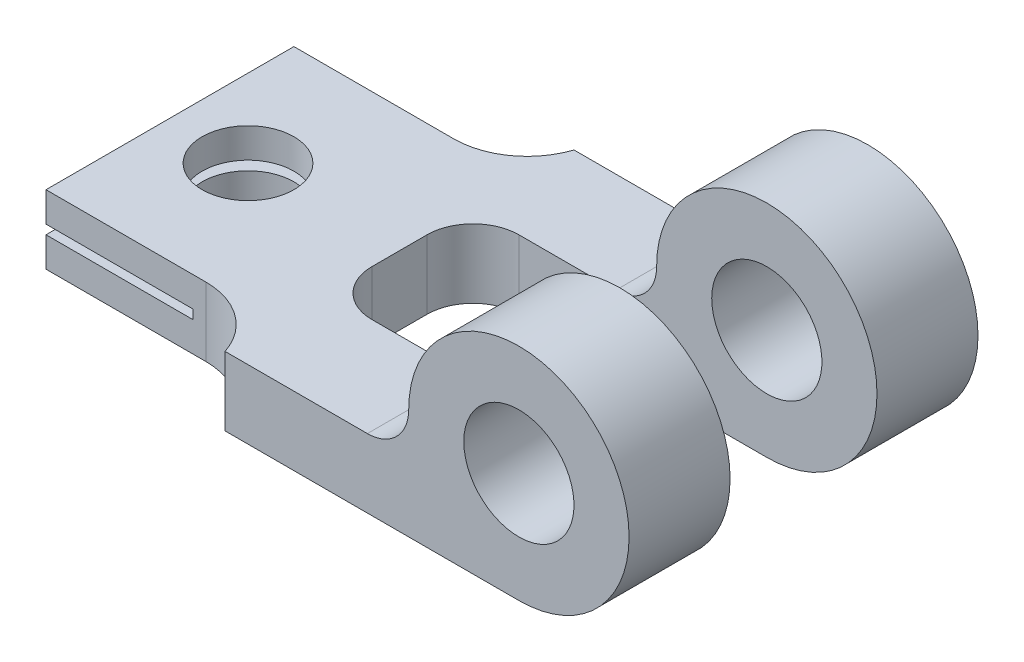
ISO-10303-21;
HEADER;
FILE_DESCRIPTION(('STEP AP214'),'2;1');
FILE_NAME('part.step','',(''),(''),'','','');
FILE_SCHEMA(('AUTOMOTIVE_DESIGN { 1 0 10303 214 1 1 1 1 }'));
ENDSEC;
DATA;
#1=APPLICATION_CONTEXT('core data for automotive mechanical design processes');
#2=APPLICATION_PROTOCOL_DEFINITION('international standard','automotive_design',2000,#1);
#3=PRODUCT_CONTEXT('',#1,'mechanical');
#4=PRODUCT('Part','Part','',(#3));
#5=PRODUCT_RELATED_PRODUCT_CATEGORY('part','',(#4));
#6=PRODUCT_DEFINITION_FORMATION('','',#4);
#7=PRODUCT_DEFINITION_CONTEXT('part definition',#1,'design');
#8=PRODUCT_DEFINITION('design','',#6,#7);
#9=PRODUCT_DEFINITION_SHAPE('','',#8);
#10=(LENGTH_UNIT() NAMED_UNIT(*) SI_UNIT(.MILLI.,.METRE.));
#11=(NAMED_UNIT(*) PLANE_ANGLE_UNIT() SI_UNIT($,.RADIAN.));
#12=(NAMED_UNIT(*) SI_UNIT($,.STERADIAN.) SOLID_ANGLE_UNIT());
#13=UNCERTAINTY_MEASURE_WITH_UNIT(LENGTH_MEASURE(1.E-05),#10,'distance_accuracy_value','');
#14=(GEOMETRIC_REPRESENTATION_CONTEXT(3) GLOBAL_UNCERTAINTY_ASSIGNED_CONTEXT((#13)) GLOBAL_UNIT_ASSIGNED_CONTEXT((#10,
#11,#12)) REPRESENTATION_CONTEXT('',''));
#15=CARTESIAN_POINT('',(0.,0.,0.));
#16=DIRECTION('',(0.,0.,1.));
#17=DIRECTION('',(1.,0.,0.));
#18=AXIS2_PLACEMENT_3D('',#15,#16,#17);
#19=CARTESIAN_POINT('',(0.,0.,27.));
#20=DIRECTION('',(-1.,0.,0.));
#21=DIRECTION('',(0.,-1.,0.));
#22=AXIS2_PLACEMENT_3D('',#19,#20,#21);
#23=PLANE('',#22);
#24=DIRECTION('',(0.,0.,-1.));
#25=VECTOR('',#24,1.);
#26=CARTESIAN_POINT('',(0.,0.,27.));
#27=LINE('',#26,#25);
#28=CARTESIAN_POINT('',(0.,0.,6.));
#29=VERTEX_POINT('',#28);
#30=CARTESIAN_POINT('',(0.,0.,-6.));
#31=VERTEX_POINT('',#30);
#32=EDGE_CURVE('E240',#29,#31,#27,.T.);
#33=ORIENTED_EDGE('',*,*,#32,.T.);
#34=DIRECTION('',(0.,1.,0.));
#35=VECTOR('',#34,1.);
#36=CARTESIAN_POINT('',(0.,15.,-6.));
#37=LINE('',#36,#35);
#38=CARTESIAN_POINT('',(0.,15.,-6.));
#39=VERTEX_POINT('',#38);
#40=EDGE_CURVE('E219',#31,#39,#37,.T.);
#41=ORIENTED_EDGE('',*,*,#40,.T.);
#42=DIRECTION('',(0.,0.,-1.));
#43=VECTOR('',#42,1.);
#44=CARTESIAN_POINT('',(0.,15.,27.));
#45=LINE('',#44,#43);
#46=CARTESIAN_POINT('',(0.,15.,6.));
#47=VERTEX_POINT('',#46);
#48=EDGE_CURVE('E235',#47,#39,#45,.T.);
#49=ORIENTED_EDGE('',*,*,#48,.F.);
#50=DIRECTION('',(0.,1.,0.));
#51=VECTOR('',#50,1.);
#52=CARTESIAN_POINT('',(0.,0.,6.));
#53=LINE('',#52,#51);
#54=EDGE_CURVE('E211',#47,#29,#53,.F.);
#55=ORIENTED_EDGE('',*,*,#54,.T.);
#56=EDGE_LOOP('',(#33,#41,#49,#55));
#57=FACE_BOUND('',#56,.T.);
#58=ADVANCED_FACE('F41',(#57),#23,.F.);
#59=CARTESIAN_POINT('',(0.,6.49999999999999,27.));
#60=DIRECTION('',(0.,1.,0.));
#61=DIRECTION('',(-1.,0.,0.));
#62=AXIS2_PLACEMENT_3D('',#59,#60,#61);
#63=PLANE('',#62);
#64=CARTESIAN_POINT('',(-33.,6.5,0.));
#65=DIRECTION('',(0.,1.,0.));
#66=DIRECTION('',(-1.,0.,0.));
#67=AXIS2_PLACEMENT_3D('',#64,#65,#66);
#68=CIRCLE('',#67,10.);
#69=CARTESIAN_POINT('',(-43.,6.5,0.));
#70=VERTEX_POINT('',#69);
#71=EDGE_CURVE('E310',#70,#70,#68,.T.);
#72=ORIENTED_EDGE('',*,*,#71,.F.);
#73=EDGE_LOOP('',(#72));
#74=FACE_BOUND('',#73,.T.);
#75=DIRECTION('',(1.,0.,0.));
#76=VECTOR('',#75,1.);
#77=CARTESIAN_POINT('',(0.,6.49999999999999,-27.));
#78=LINE('',#77,#76);
#79=CARTESIAN_POINT('',(-50.,6.5,-27.));
#80=VERTEX_POINT('',#79);
#81=CARTESIAN_POINT('',(-18.,6.49999999999999,-27.));
#82=VERTEX_POINT('',#81);
#83=EDGE_CURVE('E309',#80,#82,#78,.T.);
#84=ORIENTED_EDGE('',*,*,#83,.F.);
#85=DIRECTION('',(0.,0.,-1.));
#86=VECTOR('',#85,1.);
#87=CARTESIAN_POINT('',(-50.,6.5,27.));
#88=LINE('',#87,#86);
#89=CARTESIAN_POINT('',(-50.,6.5,27.));
#90=VERTEX_POINT('',#89);
#91=EDGE_CURVE('E356',#90,#80,#88,.T.);
#92=ORIENTED_EDGE('',*,*,#91,.F.);
#93=DIRECTION('',(1.,0.,0.));
#94=VECTOR('',#93,1.);
#95=CARTESIAN_POINT('',(0.,6.49999999999999,27.));
#96=LINE('',#95,#94);
#97=CARTESIAN_POINT('',(-18.,6.49999999999999,27.));
#98=VERTEX_POINT('',#97);
#99=EDGE_CURVE('E311',#90,#98,#96,.T.);
#100=ORIENTED_EDGE('',*,*,#99,.T.);
#101=DIRECTION('',(0.,0.,-1.));
#102=VECTOR('',#101,1.);
#103=CARTESIAN_POINT('',(-18.,6.49999999999999,27.));
#104=LINE('',#103,#102);
#105=EDGE_CURVE('E327',#98,#82,#104,.T.);
#106=ORIENTED_EDGE('',*,*,#105,.T.);
#107=EDGE_LOOP('',(#84,#92,#100,#106));
#108=FACE_BOUND('',#107,.T.);
#109=ADVANCED_FACE('F408',(#74,#108),#63,.T.);
#110=CARTESIAN_POINT('',(-50.,0.,27.));
#111=DIRECTION('',(1.,0.,0.));
#112=DIRECTION('',(0.,0.,-1.));
#113=AXIS2_PLACEMENT_3D('',#110,#111,#112);
#114=PLANE('',#113);
#115=DIRECTION('',(0.,-1.,0.));
#116=VECTOR('',#115,1.);
#117=CARTESIAN_POINT('',(-50.,0.,-27.));
#118=LINE('',#117,#116);
#119=CARTESIAN_POINT('',(-50.,0.,-27.));
#120=VERTEX_POINT('',#119);
#121=EDGE_CURVE('E332',#80,#120,#118,.T.);
#122=ORIENTED_EDGE('',*,*,#121,.T.);
#123=DIRECTION('',(0.,0.,-1.));
#124=VECTOR('',#123,1.);
#125=CARTESIAN_POINT('',(-50.,0.,27.));
#126=LINE('',#125,#124);
#127=CARTESIAN_POINT('',(-50.,0.,27.));
#128=VERTEX_POINT('',#127);
#129=EDGE_CURVE('E354',#128,#120,#126,.T.);
#130=ORIENTED_EDGE('',*,*,#129,.F.);
#131=DIRECTION('',(0.,-1.,0.));
#132=VECTOR('',#131,1.);
#133=CARTESIAN_POINT('',(-50.,0.,27.));
#134=LINE('',#133,#132);
#135=EDGE_CURVE('E313',#90,#128,#134,.T.);
#136=ORIENTED_EDGE('',*,*,#135,.F.);
#137=ORIENTED_EDGE('',*,*,#91,.T.);
#138=EDGE_LOOP('',(#122,#130,#136,#137));
#139=FACE_BOUND('',#138,.T.);
#140=ADVANCED_FACE('F420',(#139),#114,.F.);
#141=CARTESIAN_POINT('',(0.,0.,27.));
#142=DIRECTION('',(0.,1.,0.));
#143=DIRECTION('',(0.,0.,1.));
#144=AXIS2_PLACEMENT_3D('',#141,#142,#143);
#145=PLANE('',#144);
#146=CARTESIAN_POINT('',(-33.,0.,0.));
#147=DIRECTION('',(0.,1.,0.));
#148=DIRECTION('',(-1.,0.,0.));
#149=AXIS2_PLACEMENT_3D('',#146,#147,#148);
#150=CIRCLE('',#149,10.);
#151=CARTESIAN_POINT('',(-43.,0.,0.));
#152=VERTEX_POINT('',#151);
#153=EDGE_CURVE('E301',#152,#152,#150,.T.);
#154=ORIENTED_EDGE('',*,*,#153,.T.);
#155=EDGE_LOOP('',(#154));
#156=FACE_BOUND('',#155,.T.);
#157=DIRECTION('',(1.,0.,0.));
#158=VECTOR('',#157,1.);
#159=CARTESIAN_POINT('',(0.,0.,-27.));
#160=LINE('',#159,#158);
#161=CARTESIAN_POINT('',(-15.1986841535707,0.,-27.));
#162=VERTEX_POINT('',#161);
#163=EDGE_CURVE('E334',#120,#162,#160,.T.);
#164=ORIENTED_EDGE('',*,*,#163,.T.);
#165=CARTESIAN_POINT('',(-15.1986841535707,0.,-43.));
#166=DIRECTION('',(0.,1.,0.));
#167=DIRECTION('',(0.,0.,1.));
#168=AXIS2_PLACEMENT_3D('',#165,#166,#167);
#169=CIRCLE('',#168,16.);
#170=CARTESIAN_POINT('',(0.,0.,-38.));
#171=VERTEX_POINT('',#170);
#172=EDGE_CURVE('E210',#162,#171,#169,.T.);
#173=ORIENTED_EDGE('',*,*,#172,.T.);
#174=DIRECTION('',(-1.,0.,0.));
#175=VECTOR('',#174,1.);
#176=CARTESIAN_POINT('',(0.,0.,-38.));
#177=LINE('',#176,#175);
#178=CARTESIAN_POINT('',(64.,0.,-38.));
#179=VERTEX_POINT('',#178);
#180=EDGE_CURVE('E284',#179,#171,#177,.T.);
#181=ORIENTED_EDGE('',*,*,#180,.F.);
#182=DIRECTION('',(0.,0.,1.));
#183=VECTOR('',#182,1.);
#184=CARTESIAN_POINT('',(64.,0.,-38.));
#185=LINE('',#184,#183);
#186=CARTESIAN_POINT('',(64.,0.,-16.));
#187=VERTEX_POINT('',#186);
#188=EDGE_CURVE('E283',#179,#187,#185,.T.);
#189=ORIENTED_EDGE('',*,*,#188,.T.);
#190=DIRECTION('',(-1.,0.,0.));
#191=VECTOR('',#190,1.);
#192=CARTESIAN_POINT('',(0.,0.,-16.));
#193=LINE('',#192,#191);
#194=CARTESIAN_POINT('',(10.,0.,-16.));
#195=VERTEX_POINT('',#194);
#196=EDGE_CURVE('E273',#187,#195,#193,.T.);
#197=ORIENTED_EDGE('',*,*,#196,.T.);
#198=CARTESIAN_POINT('',(10.,0.,-6.));
#199=DIRECTION('',(0.,1.,0.));
#200=DIRECTION('',(0.,0.,1.));
#201=AXIS2_PLACEMENT_3D('',#198,#199,#200);
#202=CIRCLE('',#201,10.);
#203=EDGE_CURVE('E224',#195,#31,#202,.T.);
#204=ORIENTED_EDGE('',*,*,#203,.T.);
#205=ORIENTED_EDGE('',*,*,#32,.F.);
#206=CARTESIAN_POINT('',(10.,0.,6.));
#207=DIRECTION('',(0.,1.,0.));
#208=DIRECTION('',(0.,0.,1.));
#209=AXIS2_PLACEMENT_3D('',#206,#207,#208);
#210=CIRCLE('',#209,10.);
#211=CARTESIAN_POINT('',(10.,0.,16.));
#212=VERTEX_POINT('',#211);
#213=EDGE_CURVE('E11',#29,#212,#210,.T.);
#214=ORIENTED_EDGE('',*,*,#213,.T.);
#215=DIRECTION('',(-1.,0.,0.));
#216=VECTOR('',#215,1.);
#217=CARTESIAN_POINT('',(0.,0.,16.));
#218=LINE('',#217,#216);
#219=CARTESIAN_POINT('',(64.,0.,16.));
#220=VERTEX_POINT('',#219);
#221=EDGE_CURVE('E242',#220,#212,#218,.T.);
#222=ORIENTED_EDGE('',*,*,#221,.F.);
#223=DIRECTION('',(0.,0.,-1.));
#224=VECTOR('',#223,1.);
#225=CARTESIAN_POINT('',(64.,0.,38.));
#226=LINE('',#225,#224);
#227=CARTESIAN_POINT('',(64.,0.,38.));
#228=VERTEX_POINT('',#227);
#229=EDGE_CURVE('E196',#228,#220,#226,.T.);
#230=ORIENTED_EDGE('',*,*,#229,.F.);
#231=DIRECTION('',(-1.,0.,0.));
#232=VECTOR('',#231,1.);
#233=CARTESIAN_POINT('',(0.,0.,38.));
#234=LINE('',#233,#232);
#235=CARTESIAN_POINT('',(0.,0.,38.));
#236=VERTEX_POINT('',#235);
#237=EDGE_CURVE('E182',#228,#236,#234,.T.);
#238=ORIENTED_EDGE('',*,*,#237,.T.);
#239=CARTESIAN_POINT('',(-15.1986841535707,0.,43.));
#240=DIRECTION('',(0.,1.,0.));
#241=DIRECTION('',(0.,0.,1.));
#242=AXIS2_PLACEMENT_3D('',#239,#240,#241);
#243=CIRCLE('',#242,16.);
#244=CARTESIAN_POINT('',(-15.1986841535707,0.,27.));
#245=VERTEX_POINT('',#244);
#246=EDGE_CURVE('E193',#236,#245,#243,.T.);
#247=ORIENTED_EDGE('',*,*,#246,.T.);
#248=DIRECTION('',(1.,0.,0.));
#249=VECTOR('',#248,1.);
#250=CARTESIAN_POINT('',(0.,0.,27.));
#251=LINE('',#250,#249);
#252=EDGE_CURVE('E320',#128,#245,#251,.T.);
#253=ORIENTED_EDGE('',*,*,#252,.F.);
#254=ORIENTED_EDGE('',*,*,#129,.T.);
#255=EDGE_LOOP('',(#164,#173,#181,#189,#197,#204,#205,#214,#222,#230,#238,#247,#253,#254));
#256=FACE_BOUND('',#255,.T.);
#257=ADVANCED_FACE('F194',(#156,#256),#145,.F.);
#258=CARTESIAN_POINT('',(0.,15.,27.));
#259=DIRECTION('',(0.,-1.,0.));
#260=DIRECTION('',(1.,0.,0.));
#261=AXIS2_PLACEMENT_3D('',#258,#259,#260);
#262=PLANE('',#261);
#263=CARTESIAN_POINT('',(-33.,15.,0.));
#264=DIRECTION('',(0.,1.,0.));
#265=DIRECTION('',(-1.,0.,0.));
#266=AXIS2_PLACEMENT_3D('',#263,#264,#265);
#267=CIRCLE('',#266,10.);
#268=CARTESIAN_POINT('',(-43.,15.,0.));
#269=VERTEX_POINT('',#268);
#270=EDGE_CURVE('E297',#269,#269,#267,.T.);
#271=ORIENTED_EDGE('',*,*,#270,.F.);
#272=EDGE_LOOP('',(#271));
#273=FACE_BOUND('',#272,.T.);
#274=DIRECTION('',(1.,0.,0.));
#275=VECTOR('',#274,1.);
#276=CARTESIAN_POINT('',(0.,15.,-38.));
#277=LINE('',#276,#275);
#278=CARTESIAN_POINT('',(0.,15.,-38.));
#279=VERTEX_POINT('',#278);
#280=CARTESIAN_POINT('',(31.,15.,-38.));
#281=VERTEX_POINT('',#280);
#282=EDGE_CURVE('E274',#279,#281,#277,.T.);
#283=ORIENTED_EDGE('',*,*,#282,.F.);
#284=CARTESIAN_POINT('',(-15.1986841535707,15.,-43.));
#285=DIRECTION('',(0.,-1.,0.));
#286=DIRECTION('',(1.,0.,0.));
#287=AXIS2_PLACEMENT_3D('',#284,#285,#286);
#288=CIRCLE('',#287,16.);
#289=CARTESIAN_POINT('',(-15.1986841535707,15.,-27.));
#290=VERTEX_POINT('',#289);
#291=EDGE_CURVE('E203',#279,#290,#288,.T.);
#292=ORIENTED_EDGE('',*,*,#291,.T.);
#293=DIRECTION('',(-1.,0.,0.));
#294=VECTOR('',#293,1.);
#295=CARTESIAN_POINT('',(0.,15.,-27.));
#296=LINE('',#295,#294);
#297=CARTESIAN_POINT('',(-50.,15.,-27.));
#298=VERTEX_POINT('',#297);
#299=EDGE_CURVE('E340',#290,#298,#296,.T.);
#300=ORIENTED_EDGE('',*,*,#299,.T.);
#301=DIRECTION('',(0.,0.,-1.));
#302=VECTOR('',#301,1.);
#303=CARTESIAN_POINT('',(-50.,15.,27.));
#304=LINE('',#303,#302);
#305=CARTESIAN_POINT('',(-50.,15.,27.));
#306=VERTEX_POINT('',#305);
#307=EDGE_CURVE('E238',#306,#298,#304,.T.);
#308=ORIENTED_EDGE('',*,*,#307,.F.);
#309=DIRECTION('',(-1.,0.,0.));
#310=VECTOR('',#309,1.);
#311=CARTESIAN_POINT('',(0.,15.,27.));
#312=LINE('',#311,#310);
#313=CARTESIAN_POINT('',(-15.1986841535707,15.,27.));
#314=VERTEX_POINT('',#313);
#315=EDGE_CURVE('E316',#314,#306,#312,.T.);
#316=ORIENTED_EDGE('',*,*,#315,.F.);
#317=CARTESIAN_POINT('',(-15.1986841535707,15.,43.));
#318=DIRECTION('',(0.,-1.,0.));
#319=DIRECTION('',(1.,0.,0.));
#320=AXIS2_PLACEMENT_3D('',#317,#318,#319);
#321=CIRCLE('',#320,16.);
#322=CARTESIAN_POINT('',(0.,15.,38.));
#323=VERTEX_POINT('',#322);
#324=EDGE_CURVE('E204',#314,#323,#321,.T.);
#325=ORIENTED_EDGE('',*,*,#324,.T.);
#326=DIRECTION('',(1.,0.,0.));
#327=VECTOR('',#326,1.);
#328=CARTESIAN_POINT('',(0.,15.,38.));
#329=LINE('',#328,#327);
#330=CARTESIAN_POINT('',(31.,15.,38.));
#331=VERTEX_POINT('',#330);
#332=EDGE_CURVE('E190',#323,#331,#329,.T.);
#333=ORIENTED_EDGE('',*,*,#332,.T.);
#334=DIRECTION('',(0.,0.,-1.));
#335=VECTOR('',#334,1.);
#336=CARTESIAN_POINT('',(31.,15.,38.));
#337=LINE('',#336,#335);
#338=CARTESIAN_POINT('',(31.,15.,16.));
#339=VERTEX_POINT('',#338);
#340=EDGE_CURVE('E256',#331,#339,#337,.T.);
#341=ORIENTED_EDGE('',*,*,#340,.T.);
#342=DIRECTION('',(1.,0.,0.));
#343=VECTOR('',#342,1.);
#344=CARTESIAN_POINT('',(0.,15.,16.));
#345=LINE('',#344,#343);
#346=CARTESIAN_POINT('',(10.,15.,16.));
#347=VERTEX_POINT('',#346);
#348=EDGE_CURVE('E188',#347,#339,#345,.T.);
#349=ORIENTED_EDGE('',*,*,#348,.F.);
#350=CARTESIAN_POINT('',(10.,15.,6.));
#351=DIRECTION('',(0.,-1.,0.));
#352=DIRECTION('',(1.,0.,0.));
#353=AXIS2_PLACEMENT_3D('',#350,#351,#352);
#354=CIRCLE('',#353,10.);
#355=EDGE_CURVE('E47',#347,#47,#354,.T.);
#356=ORIENTED_EDGE('',*,*,#355,.T.);
#357=ORIENTED_EDGE('',*,*,#48,.T.);
#358=CARTESIAN_POINT('',(10.,15.,-6.));
#359=DIRECTION('',(0.,-1.,0.));
#360=DIRECTION('',(1.,0.,0.));
#361=AXIS2_PLACEMENT_3D('',#358,#359,#360);
#362=CIRCLE('',#361,10.);
#363=CARTESIAN_POINT('',(10.,15.,-16.));
#364=VERTEX_POINT('',#363);
#365=EDGE_CURVE('E222',#39,#364,#362,.T.);
#366=ORIENTED_EDGE('',*,*,#365,.T.);
#367=DIRECTION('',(1.,0.,0.));
#368=VECTOR('',#367,1.);
#369=CARTESIAN_POINT('',(0.,15.,-16.));
#370=LINE('',#369,#368);
#371=CARTESIAN_POINT('',(31.,15.,-16.));
#372=VERTEX_POINT('',#371);
#373=EDGE_CURVE('E267',#364,#372,#370,.T.);
#374=ORIENTED_EDGE('',*,*,#373,.T.);
#375=DIRECTION('',(0.,0.,1.));
#376=VECTOR('',#375,1.);
#377=CARTESIAN_POINT('',(31.,15.,-38.));
#378=LINE('',#377,#376);
#379=EDGE_CURVE('E300',#281,#372,#378,.T.);
#380=ORIENTED_EDGE('',*,*,#379,.F.);
#381=EDGE_LOOP('',(#283,#292,#300,#308,#316,#325,#333,#341,#349,#356,#357,#366,#374,#380));
#382=FACE_BOUND('',#381,.T.);
#383=ADVANCED_FACE('F233',(#273,#382),#262,.F.);
#384=CARTESIAN_POINT('',(-50.,0.,27.));
#385=DIRECTION('',(-1.,0.,0.));
#386=DIRECTION('',(0.,0.,1.));
#387=AXIS2_PLACEMENT_3D('',#384,#385,#386);
#388=PLANE('',#387);
#389=DIRECTION('',(0.,1.,0.));
#390=VECTOR('',#389,1.);
#391=CARTESIAN_POINT('',(-50.,0.,-27.));
#392=LINE('',#391,#390);
#393=CARTESIAN_POINT('',(-50.,8.49999999999999,-27.));
#394=VERTEX_POINT('',#393);
#395=EDGE_CURVE('E339',#394,#298,#392,.T.);
#396=ORIENTED_EDGE('',*,*,#395,.F.);
#397=DIRECTION('',(0.,0.,-1.));
#398=VECTOR('',#397,1.);
#399=CARTESIAN_POINT('',(-50.,8.49999999999999,27.));
#400=LINE('',#399,#398);
#401=CARTESIAN_POINT('',(-50.,8.49999999999999,27.));
#402=VERTEX_POINT('',#401);
#403=EDGE_CURVE('E347',#402,#394,#400,.T.);
#404=ORIENTED_EDGE('',*,*,#403,.F.);
#405=DIRECTION('',(0.,1.,0.));
#406=VECTOR('',#405,1.);
#407=CARTESIAN_POINT('',(-50.,0.,27.));
#408=LINE('',#407,#406);
#409=EDGE_CURVE('E322',#402,#306,#408,.T.);
#410=ORIENTED_EDGE('',*,*,#409,.T.);
#411=ORIENTED_EDGE('',*,*,#307,.T.);
#412=EDGE_LOOP('',(#396,#404,#410,#411));
#413=FACE_BOUND('',#412,.T.);
#414=ADVANCED_FACE('F515',(#413),#388,.T.);
#415=CARTESIAN_POINT('',(0.,8.5,27.));
#416=DIRECTION('',(0.,-1.,0.));
#417=DIRECTION('',(1.,0.,0.));
#418=AXIS2_PLACEMENT_3D('',#415,#416,#417);
#419=PLANE('',#418);
#420=CARTESIAN_POINT('',(-33.,8.5,0.));
#421=DIRECTION('',(0.,-1.,0.));
#422=DIRECTION('',(1.,0.,0.));
#423=AXIS2_PLACEMENT_3D('',#420,#421,#422);
#424=CIRCLE('',#423,10.);
#425=CARTESIAN_POINT('',(-23.,8.5,0.));
#426=VERTEX_POINT('',#425);
#427=EDGE_CURVE('E302',#426,#426,#424,.T.);
#428=ORIENTED_EDGE('',*,*,#427,.F.);
#429=EDGE_LOOP('',(#428));
#430=FACE_BOUND('',#429,.T.);
#431=DIRECTION('',(-1.,0.,0.));
#432=VECTOR('',#431,1.);
#433=CARTESIAN_POINT('',(0.,8.5,-27.));
#434=LINE('',#433,#432);
#435=CARTESIAN_POINT('',(-18.,8.5,-27.));
#436=VERTEX_POINT('',#435);
#437=EDGE_CURVE('E345',#436,#394,#434,.T.);
#438=ORIENTED_EDGE('',*,*,#437,.F.);
#439=DIRECTION('',(0.,0.,-1.));
#440=VECTOR('',#439,1.);
#441=CARTESIAN_POINT('',(-18.,8.5,27.));
#442=LINE('',#441,#440);
#443=CARTESIAN_POINT('',(-18.,8.5,27.));
#444=VERTEX_POINT('',#443);
#445=EDGE_CURVE('E350',#444,#436,#442,.T.);
#446=ORIENTED_EDGE('',*,*,#445,.F.);
#447=DIRECTION('',(-1.,0.,0.));
#448=VECTOR('',#447,1.);
#449=CARTESIAN_POINT('',(0.,8.5,27.));
#450=LINE('',#449,#448);
#451=EDGE_CURVE('E321',#444,#402,#450,.T.);
#452=ORIENTED_EDGE('',*,*,#451,.T.);
#453=ORIENTED_EDGE('',*,*,#403,.T.);
#454=EDGE_LOOP('',(#438,#446,#452,#453));
#455=FACE_BOUND('',#454,.T.);
#456=ADVANCED_FACE('F586',(#430,#455),#419,.T.);
#457=CARTESIAN_POINT('',(-18.,0.,27.));
#458=DIRECTION('',(-1.,0.,0.));
#459=DIRECTION('',(0.,0.,1.));
#460=AXIS2_PLACEMENT_3D('',#457,#458,#459);
#461=PLANE('',#460);
#462=DIRECTION('',(0.,1.,0.));
#463=VECTOR('',#462,1.);
#464=CARTESIAN_POINT('',(-18.,0.,-27.));
#465=LINE('',#464,#463);
#466=EDGE_CURVE('E314',#82,#436,#465,.T.);
#467=ORIENTED_EDGE('',*,*,#466,.F.);
#468=ORIENTED_EDGE('',*,*,#105,.F.);
#469=DIRECTION('',(0.,1.,0.));
#470=VECTOR('',#469,1.);
#471=CARTESIAN_POINT('',(-18.,0.,27.));
#472=LINE('',#471,#470);
#473=EDGE_CURVE('E326',#98,#444,#472,.T.);
#474=ORIENTED_EDGE('',*,*,#473,.T.);
#475=ORIENTED_EDGE('',*,*,#445,.T.);
#476=EDGE_LOOP('',(#467,#468,#474,#475));
#477=FACE_BOUND('',#476,.T.);
#478=ADVANCED_FACE('F573',(#477),#461,.T.);
#479=CARTESIAN_POINT('',(0.,0.,27.));
#480=DIRECTION('',(0.,0.,1.));
#481=DIRECTION('',(1.,0.,0.));
#482=AXIS2_PLACEMENT_3D('',#479,#480,#481);
#483=PLANE('',#482);
#484=ORIENTED_EDGE('',*,*,#252,.T.);
#485=DIRECTION('',(0.,-1.,0.));
#486=VECTOR('',#485,1.);
#487=CARTESIAN_POINT('',(-15.1986841535707,15.,27.));
#488=LINE('',#487,#486);
#489=EDGE_CURVE('E202',#245,#314,#488,.F.);
#490=ORIENTED_EDGE('',*,*,#489,.T.);
#491=ORIENTED_EDGE('',*,*,#315,.T.);
#492=ORIENTED_EDGE('',*,*,#409,.F.);
#493=ORIENTED_EDGE('',*,*,#451,.F.);
#494=ORIENTED_EDGE('',*,*,#473,.F.);
#495=ORIENTED_EDGE('',*,*,#99,.F.);
#496=ORIENTED_EDGE('',*,*,#135,.T.);
#497=EDGE_LOOP('',(#484,#490,#491,#492,#493,#494,#495,#496));
#498=FACE_BOUND('',#497,.T.);
#499=ADVANCED_FACE('F566',(#498),#483,.T.);
#500=CARTESIAN_POINT('',(0.,0.,-27.));
#501=DIRECTION('',(0.,0.,1.));
#502=DIRECTION('',(1.,0.,0.));
#503=AXIS2_PLACEMENT_3D('',#500,#501,#502);
#504=PLANE('',#503);
#505=ORIENTED_EDGE('',*,*,#299,.F.);
#506=DIRECTION('',(0.,1.,0.));
#507=VECTOR('',#506,1.);
#508=CARTESIAN_POINT('',(-15.1986841535707,0.,-27.));
#509=LINE('',#508,#507);
#510=EDGE_CURVE('E209',#290,#162,#509,.F.);
#511=ORIENTED_EDGE('',*,*,#510,.T.);
#512=ORIENTED_EDGE('',*,*,#163,.F.);
#513=ORIENTED_EDGE('',*,*,#121,.F.);
#514=ORIENTED_EDGE('',*,*,#83,.T.);
#515=ORIENTED_EDGE('',*,*,#466,.T.);
#516=ORIENTED_EDGE('',*,*,#437,.T.);
#517=ORIENTED_EDGE('',*,*,#395,.T.);
#518=EDGE_LOOP('',(#505,#511,#512,#513,#514,#515,#516,#517));
#519=FACE_BOUND('',#518,.T.);
#520=ADVANCED_FACE('F366',(#519),#504,.F.);
#521=CARTESIAN_POINT('',(-33.,0.,0.));
#522=DIRECTION('',(0.,1.,0.));
#523=DIRECTION('',(-1.,0.,0.));
#524=AXIS2_PLACEMENT_3D('',#521,#522,#523);
#525=CYLINDRICAL_SURFACE('',#524,10.);
#526=ORIENTED_EDGE('',*,*,#427,.T.);
#527=EDGE_LOOP('',(#526));
#528=FACE_BOUND('',#527,.T.);
#529=ORIENTED_EDGE('',*,*,#270,.T.);
#530=EDGE_LOOP('',(#529));
#531=FACE_BOUND('',#530,.T.);
#532=ADVANCED_FACE('F564',(#528,#531),#525,.F.);
#533=ORIENTED_EDGE('',*,*,#71,.T.);
#534=EDGE_LOOP('',(#533));
#535=FACE_BOUND('',#534,.T.);
#536=ORIENTED_EDGE('',*,*,#153,.F.);
#537=EDGE_LOOP('',(#536));
#538=FACE_BOUND('',#537,.T.);
#539=ADVANCED_FACE('F560',(#535,#538),#525,.F.);
#540=CARTESIAN_POINT('',(31.,24.,-38.));
#541=DIRECTION('',(0.,0.,-1.));
#542=DIRECTION('',(-1.,0.,0.));
#543=AXIS2_PLACEMENT_3D('',#540,#541,#542);
#544=PLANE('',#543);
#545=DIRECTION('',(0.,1.,0.));
#546=VECTOR('',#545,1.);
#547=CARTESIAN_POINT('',(0.,0.,-38.));
#548=LINE('',#547,#546);
#549=EDGE_CURVE('E272',#171,#279,#548,.T.);
#550=ORIENTED_EDGE('',*,*,#549,.T.);
#551=ORIENTED_EDGE('',*,*,#282,.T.);
#552=CARTESIAN_POINT('',(31.,24.,-38.));
#553=DIRECTION('',(0.,0.,1.));
#554=DIRECTION('',(-1.,0.,0.));
#555=AXIS2_PLACEMENT_3D('',#552,#553,#554);
#556=CIRCLE('',#555,9.00000000000001);
#557=CARTESIAN_POINT('',(40.,24.,-38.));
#558=VERTEX_POINT('',#557);
#559=EDGE_CURVE('E280',#281,#558,#556,.T.);
#560=ORIENTED_EDGE('',*,*,#559,.T.);
#561=CARTESIAN_POINT('',(64.,24.,-38.));
#562=DIRECTION('',(0.,0.,-1.));
#563=DIRECTION('',(-1.,0.,0.));
#564=AXIS2_PLACEMENT_3D('',#561,#562,#563);
#565=CIRCLE('',#564,24.);
#566=EDGE_CURVE('E276',#558,#179,#565,.T.);
#567=ORIENTED_EDGE('',*,*,#566,.T.);
#568=ORIENTED_EDGE('',*,*,#180,.T.);
#569=EDGE_LOOP('',(#550,#551,#560,#567,#568));
#570=FACE_BOUND('',#569,.T.);
#571=CARTESIAN_POINT('',(64.,24.,-38.));
#572=DIRECTION('',(0.,0.,-1.));
#573=DIRECTION('',(-1.,0.,0.));
#574=AXIS2_PLACEMENT_3D('',#571,#572,#573);
#575=CIRCLE('',#574,12.);
#576=CARTESIAN_POINT('',(52.,24.,-38.));
#577=VERTEX_POINT('',#576);
#578=EDGE_CURVE('E262',#577,#577,#575,.T.);
#579=ORIENTED_EDGE('',*,*,#578,.F.);
#580=EDGE_LOOP('',(#579));
#581=FACE_BOUND('',#580,.T.);
#582=ADVANCED_FACE('F374',(#570,#581),#544,.T.);
#583=CARTESIAN_POINT('',(31.,24.,-16.));
#584=DIRECTION('',(0.,0.,-1.));
#585=DIRECTION('',(-1.,0.,0.));
#586=AXIS2_PLACEMENT_3D('',#583,#584,#585);
#587=PLANE('',#586);
#588=ORIENTED_EDGE('',*,*,#373,.F.);
#589=DIRECTION('',(0.,1.,0.));
#590=VECTOR('',#589,1.);
#591=CARTESIAN_POINT('',(10.,0.,-16.));
#592=LINE('',#591,#590);
#593=EDGE_CURVE('E218',#364,#195,#592,.F.);
#594=ORIENTED_EDGE('',*,*,#593,.T.);
#595=ORIENTED_EDGE('',*,*,#196,.F.);
#596=CARTESIAN_POINT('',(64.,24.,-16.));
#597=DIRECTION('',(0.,0.,-1.));
#598=DIRECTION('',(-1.,0.,0.));
#599=AXIS2_PLACEMENT_3D('',#596,#597,#598);
#600=CIRCLE('',#599,24.);
#601=CARTESIAN_POINT('',(40.,24.,-16.));
#602=VERTEX_POINT('',#601);
#603=EDGE_CURVE('E287',#602,#187,#600,.T.);
#604=ORIENTED_EDGE('',*,*,#603,.F.);
#605=CARTESIAN_POINT('',(31.,24.,-16.));
#606=DIRECTION('',(0.,0.,1.));
#607=DIRECTION('',(-1.,0.,0.));
#608=AXIS2_PLACEMENT_3D('',#605,#606,#607);
#609=CIRCLE('',#608,9.00000000000001);
#610=EDGE_CURVE('E286',#372,#602,#609,.T.);
#611=ORIENTED_EDGE('',*,*,#610,.F.);
#612=EDGE_LOOP('',(#588,#594,#595,#604,#611));
#613=FACE_BOUND('',#612,.T.);
#614=CARTESIAN_POINT('',(64.,24.,-16.));
#615=DIRECTION('',(0.,0.,-1.));
#616=DIRECTION('',(-1.,0.,0.));
#617=AXIS2_PLACEMENT_3D('',#614,#615,#616);
#618=CIRCLE('',#617,12.);
#619=CARTESIAN_POINT('',(52.,24.,-16.));
#620=VERTEX_POINT('',#619);
#621=EDGE_CURVE('E263',#620,#620,#618,.T.);
#622=ORIENTED_EDGE('',*,*,#621,.T.);
#623=EDGE_LOOP('',(#622));
#624=FACE_BOUND('',#623,.T.);
#625=ADVANCED_FACE('F387',(#613,#624),#587,.F.);
#626=CARTESIAN_POINT('',(31.,24.,-38.));
#627=DIRECTION('',(0.,0.,1.));
#628=DIRECTION('',(1.,0.,0.));
#629=AXIS2_PLACEMENT_3D('',#626,#627,#628);
#630=CYLINDRICAL_SURFACE('',#629,9.00000000000001);
#631=ORIENTED_EDGE('',*,*,#610,.T.);
#632=DIRECTION('',(0.,0.,1.));
#633=VECTOR('',#632,1.);
#634=CARTESIAN_POINT('',(40.,24.,-38.));
#635=LINE('',#634,#633);
#636=EDGE_CURVE('E295',#558,#602,#635,.T.);
#637=ORIENTED_EDGE('',*,*,#636,.F.);
#638=ORIENTED_EDGE('',*,*,#559,.F.);
#639=ORIENTED_EDGE('',*,*,#379,.T.);
#640=EDGE_LOOP('',(#631,#637,#638,#639));
#641=FACE_BOUND('',#640,.T.);
#642=ADVANCED_FACE('F393',(#641),#630,.F.);
#643=CARTESIAN_POINT('',(64.,24.,-38.));
#644=DIRECTION('',(0.,0.,1.));
#645=DIRECTION('',(1.,0.,0.));
#646=AXIS2_PLACEMENT_3D('',#643,#644,#645);
#647=CYLINDRICAL_SURFACE('',#646,24.);
#648=ORIENTED_EDGE('',*,*,#603,.T.);
#649=ORIENTED_EDGE('',*,*,#188,.F.);
#650=ORIENTED_EDGE('',*,*,#566,.F.);
#651=ORIENTED_EDGE('',*,*,#636,.T.);
#652=EDGE_LOOP('',(#648,#649,#650,#651));
#653=FACE_BOUND('',#652,.T.);
#654=ADVANCED_FACE('F396',(#653),#647,.T.);
#655=CARTESIAN_POINT('',(64.,24.,-38.));
#656=DIRECTION('',(0.,0.,1.));
#657=DIRECTION('',(1.,0.,0.));
#658=AXIS2_PLACEMENT_3D('',#655,#656,#657);
#659=CYLINDRICAL_SURFACE('',#658,12.);
#660=ORIENTED_EDGE('',*,*,#578,.T.);
#661=EDGE_LOOP('',(#660));
#662=FACE_BOUND('',#661,.T.);
#663=ORIENTED_EDGE('',*,*,#621,.F.);
#664=EDGE_LOOP('',(#663));
#665=FACE_BOUND('',#664,.T.);
#666=ADVANCED_FACE('F397',(#662,#665),#659,.F.);
#667=CARTESIAN_POINT('',(64.,24.,38.));
#668=DIRECTION('',(0.,0.,-1.));
#669=DIRECTION('',(-1.,0.,0.));
#670=AXIS2_PLACEMENT_3D('',#667,#668,#669);
#671=CYLINDRICAL_SURFACE('',#670,24.);
#672=CARTESIAN_POINT('',(64.,24.,16.));
#673=DIRECTION('',(0.,0.,-1.));
#674=DIRECTION('',(-1.,0.,0.));
#675=AXIS2_PLACEMENT_3D('',#672,#673,#674);
#676=CIRCLE('',#675,24.);
#677=CARTESIAN_POINT('',(40.,24.,16.));
#678=VERTEX_POINT('',#677);
#679=EDGE_CURVE('E246',#678,#220,#676,.T.);
#680=ORIENTED_EDGE('',*,*,#679,.F.);
#681=DIRECTION('',(0.,0.,-1.));
#682=VECTOR('',#681,1.);
#683=CARTESIAN_POINT('',(40.,24.,38.));
#684=LINE('',#683,#682);
#685=CARTESIAN_POINT('',(40.,24.,38.));
#686=VERTEX_POINT('',#685);
#687=EDGE_CURVE('E264',#686,#678,#684,.T.);
#688=ORIENTED_EDGE('',*,*,#687,.F.);
#689=CARTESIAN_POINT('',(64.,24.,38.));
#690=DIRECTION('',(0.,0.,-1.));
#691=DIRECTION('',(-1.,0.,0.));
#692=AXIS2_PLACEMENT_3D('',#689,#690,#691);
#693=CIRCLE('',#692,24.);
#694=EDGE_CURVE('E200',#686,#228,#693,.T.);
#695=ORIENTED_EDGE('',*,*,#694,.T.);
#696=ORIENTED_EDGE('',*,*,#229,.T.);
#697=EDGE_LOOP('',(#680,#688,#695,#696));
#698=FACE_BOUND('',#697,.T.);
#699=ADVANCED_FACE('F404',(#698),#671,.T.);
#700=CARTESIAN_POINT('',(31.,24.,38.));
#701=DIRECTION('',(0.,0.,-1.));
#702=DIRECTION('',(-1.,0.,0.));
#703=AXIS2_PLACEMENT_3D('',#700,#701,#702);
#704=CYLINDRICAL_SURFACE('',#703,9.00000000000001);
#705=CARTESIAN_POINT('',(31.,24.,16.));
#706=DIRECTION('',(0.,0.,1.));
#707=DIRECTION('',(-1.,0.,0.));
#708=AXIS2_PLACEMENT_3D('',#705,#706,#707);
#709=CIRCLE('',#708,9.00000000000001);
#710=EDGE_CURVE('E248',#339,#678,#709,.T.);
#711=ORIENTED_EDGE('',*,*,#710,.F.);
#712=ORIENTED_EDGE('',*,*,#340,.F.);
#713=CARTESIAN_POINT('',(31.,24.,38.));
#714=DIRECTION('',(0.,0.,1.));
#715=DIRECTION('',(-1.,0.,0.));
#716=AXIS2_PLACEMENT_3D('',#713,#714,#715);
#717=CIRCLE('',#716,9.00000000000001);
#718=EDGE_CURVE('E648',#331,#686,#717,.T.);
#719=ORIENTED_EDGE('',*,*,#718,.T.);
#720=ORIENTED_EDGE('',*,*,#687,.T.);
#721=EDGE_LOOP('',(#711,#712,#719,#720));
#722=FACE_BOUND('',#721,.T.);
#723=ADVANCED_FACE('F483',(#722),#704,.F.);
#724=CARTESIAN_POINT('',(31.,24.,38.));
#725=DIRECTION('',(0.,0.,1.));
#726=DIRECTION('',(-1.,0.,0.));
#727=AXIS2_PLACEMENT_3D('',#724,#725,#726);
#728=PLANE('',#727);
#729=CARTESIAN_POINT('',(64.,24.,38.));
#730=DIRECTION('',(0.,0.,-1.));
#731=DIRECTION('',(-1.,0.,0.));
#732=AXIS2_PLACEMENT_3D('',#729,#730,#731);
#733=CIRCLE('',#732,12.);
#734=CARTESIAN_POINT('',(52.,24.,38.));
#735=VERTEX_POINT('',#734);
#736=EDGE_CURVE('E250',#735,#735,#733,.T.);
#737=ORIENTED_EDGE('',*,*,#736,.T.);
#738=EDGE_LOOP('',(#737));
#739=FACE_BOUND('',#738,.T.);
#740=DIRECTION('',(0.,1.,0.));
#741=VECTOR('',#740,1.);
#742=CARTESIAN_POINT('',(0.,0.,38.));
#743=LINE('',#742,#741);
#744=EDGE_CURVE('E177',#236,#323,#743,.T.);
#745=ORIENTED_EDGE('',*,*,#744,.F.);
#746=ORIENTED_EDGE('',*,*,#237,.F.);
#747=ORIENTED_EDGE('',*,*,#694,.F.);
#748=ORIENTED_EDGE('',*,*,#718,.F.);
#749=ORIENTED_EDGE('',*,*,#332,.F.);
#750=EDGE_LOOP('',(#745,#746,#747,#748,#749));
#751=FACE_BOUND('',#750,.T.);
#752=ADVANCED_FACE('F181',(#739,#751),#728,.T.);
#753=CARTESIAN_POINT('',(31.,24.,16.));
#754=DIRECTION('',(0.,0.,1.));
#755=DIRECTION('',(-1.,0.,0.));
#756=AXIS2_PLACEMENT_3D('',#753,#754,#755);
#757=PLANE('',#756);
#758=CARTESIAN_POINT('',(64.,24.,16.));
#759=DIRECTION('',(0.,0.,-1.));
#760=DIRECTION('',(-1.,0.,0.));
#761=AXIS2_PLACEMENT_3D('',#758,#759,#760);
#762=CIRCLE('',#761,12.);
#763=CARTESIAN_POINT('',(52.,24.,16.));
#764=VERTEX_POINT('',#763);
#765=EDGE_CURVE('E255',#764,#764,#762,.T.);
#766=ORIENTED_EDGE('',*,*,#765,.F.);
#767=EDGE_LOOP('',(#766));
#768=FACE_BOUND('',#767,.T.);
#769=ORIENTED_EDGE('',*,*,#221,.T.);
#770=DIRECTION('',(0.,1.,0.));
#771=VECTOR('',#770,1.);
#772=CARTESIAN_POINT('',(10.,15.,16.));
#773=LINE('',#772,#771);
#774=EDGE_CURVE('E221',#212,#347,#773,.T.);
#775=ORIENTED_EDGE('',*,*,#774,.T.);
#776=ORIENTED_EDGE('',*,*,#348,.T.);
#777=ORIENTED_EDGE('',*,*,#710,.T.);
#778=ORIENTED_EDGE('',*,*,#679,.T.);
#779=EDGE_LOOP('',(#769,#775,#776,#777,#778));
#780=FACE_BOUND('',#779,.T.);
#781=ADVANCED_FACE('F241',(#768,#780),#757,.F.);
#782=CARTESIAN_POINT('',(64.,24.,38.));
#783=DIRECTION('',(0.,0.,-1.));
#784=DIRECTION('',(-1.,0.,0.));
#785=AXIS2_PLACEMENT_3D('',#782,#783,#784);
#786=CYLINDRICAL_SURFACE('',#785,12.);
#787=ORIENTED_EDGE('',*,*,#736,.F.);
#788=EDGE_LOOP('',(#787));
#789=FACE_BOUND('',#788,.T.);
#790=ORIENTED_EDGE('',*,*,#765,.T.);
#791=EDGE_LOOP('',(#790));
#792=FACE_BOUND('',#791,.T.);
#793=ADVANCED_FACE('F427',(#789,#792),#786,.F.);
#794=CARTESIAN_POINT('',(-15.1986841535707,0.,43.));
#795=DIRECTION('',(0.,1.,0.));
#796=DIRECTION('',(-1.,0.,0.));
#797=AXIS2_PLACEMENT_3D('',#794,#795,#796);
#798=CYLINDRICAL_SURFACE('',#797,16.);
#799=ORIENTED_EDGE('',*,*,#246,.F.);
#800=ORIENTED_EDGE('',*,*,#744,.T.);
#801=ORIENTED_EDGE('',*,*,#324,.F.);
#802=ORIENTED_EDGE('',*,*,#489,.F.);
#803=EDGE_LOOP('',(#799,#800,#801,#802));
#804=FACE_BOUND('',#803,.T.);
#805=ADVANCED_FACE('F201',(#804),#798,.F.);
#806=CARTESIAN_POINT('',(-15.1986841535707,0.,-43.));
#807=DIRECTION('',(0.,1.,0.));
#808=DIRECTION('',(-1.,0.,0.));
#809=AXIS2_PLACEMENT_3D('',#806,#807,#808);
#810=CYLINDRICAL_SURFACE('',#809,16.);
#811=ORIENTED_EDGE('',*,*,#172,.F.);
#812=ORIENTED_EDGE('',*,*,#510,.F.);
#813=ORIENTED_EDGE('',*,*,#291,.F.);
#814=ORIENTED_EDGE('',*,*,#549,.F.);
#815=EDGE_LOOP('',(#811,#812,#813,#814));
#816=FACE_BOUND('',#815,.T.);
#817=ADVANCED_FACE('F373',(#816),#810,.F.);
#818=CARTESIAN_POINT('',(10.,0.,-6.));
#819=DIRECTION('',(0.,-1.,0.));
#820=DIRECTION('',(1.,0.,0.));
#821=AXIS2_PLACEMENT_3D('',#818,#819,#820);
#822=CYLINDRICAL_SURFACE('',#821,10.);
#823=ORIENTED_EDGE('',*,*,#203,.F.);
#824=ORIENTED_EDGE('',*,*,#593,.F.);
#825=ORIENTED_EDGE('',*,*,#365,.F.);
#826=ORIENTED_EDGE('',*,*,#40,.F.);
#827=EDGE_LOOP('',(#823,#824,#825,#826));
#828=FACE_BOUND('',#827,.T.);
#829=ADVANCED_FACE('F394',(#828),#822,.F.);
#830=CARTESIAN_POINT('',(10.,24.,6.));
#831=DIRECTION('',(0.,-1.,0.));
#832=DIRECTION('',(1.,0.,0.));
#833=AXIS2_PLACEMENT_3D('',#830,#831,#832);
#834=CYLINDRICAL_SURFACE('',#833,10.);
#835=ORIENTED_EDGE('',*,*,#213,.F.);
#836=ORIENTED_EDGE('',*,*,#54,.F.);
#837=ORIENTED_EDGE('',*,*,#355,.F.);
#838=ORIENTED_EDGE('',*,*,#774,.F.);
#839=EDGE_LOOP('',(#835,#836,#837,#838));
#840=FACE_BOUND('',#839,.T.);
#841=ADVANCED_FACE('F43',(#840),#834,.F.);
#842=CLOSED_SHELL('',(#58,#109,#140,#257,#383,#414,#456,#478,#499,#520,#532,#539,#582,#625,#642,
#654,#666,#699,#723,#752,#781,#793,#805,#817,#829,#841));
#843=MANIFOLD_SOLID_BREP('B2',#842);
#844=ADVANCED_BREP_SHAPE_REPRESENTATION('',(#18,#843),#14);
#845=SHAPE_DEFINITION_REPRESENTATION(#9,#844);
ENDSEC;
END-ISO-10303-21;
